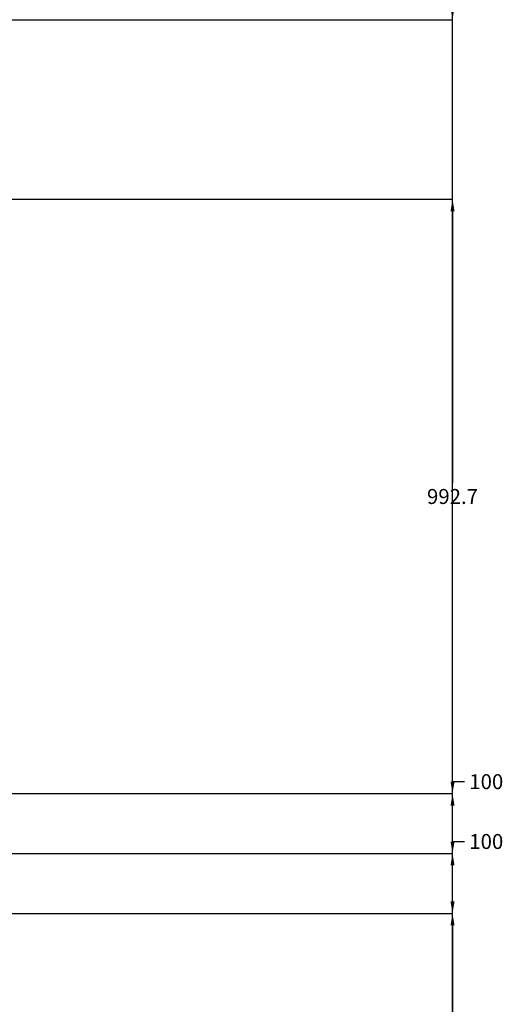
# Model space of a CAD drawing. Units: millimetres. Extents: x -692 to 9639, y -141 to 10345.
# Tile 9 of 19: x 8831 to 9639, y 1504 to 3148. Entities that reach past the tile are written whole.
import ezdxf

# ---------------------------------------------------------------- set-up
doc = ezdxf.new("R2010")
doc.units = ezdxf.units.MM
doc.header["$MEASUREMENT"] = 0
doc.layers.add('A-ANNO-DIMS', color=2, linetype='Continuous', lineweight=18)
doc.styles.get("Standard").update_dxf_attribs({"font": 'arial.ttf'})
doc.dimstyles.get("Standard").update_dxf_attribs({"dimtxt": 25, "dimasz": 20, "dimexe": 0.18, "dimexo": 10, "dimgap": 10, "dimtad": 0, "dimtih": 1, "dimtoh": 1, "dimdec": 0, "dimzin": 0, "dimdsep": 46, "dimtxsty": 'Standard', "dimcen": 10, "dimadec": 0, "dimazin": 0, "dimtfac": 1, "dimtdec": 0, "dimtofl": 0, "dimtmove": 0, "dimatfit": 3, "dimfxl": 1, "dimtolj": 1, "dimtzin": 0, "dimarcsym": 0})

# ---------------------------------------------------------------- blocks, each defined once
blk = doc.blocks.new('*D9')
at = {"layer": 'A-ANNO-DIMS', "color": 0, "lineweight": -2, "transparency": 16777216}
for p, q in [((8501.5, 8848.8), (9553.9, 8848.8)), ((9553.7, 8828.8), (9553.7, 4874.9)), ((9553.7, 875.6), (9553.7, 4829.4)), ((9083.7, 855.6), (9553.9, 855.6))]:
    blk.add_line(p, q, dxfattribs=at)
at = {"layer": 'A-ANNO-DIMS', "color": 0, "lineweight": -3, "transparency": 16777216}
for points in [[(9550.4, 8828.8), (9557.1, 8828.8), (9553.7, 8848.8)], [(9550.4, 875.6), (9557.1, 875.6), (9553.7, 855.6)]]:
    blk.add_solid(points, dxfattribs=at)
at = {"layer": 'Defpoints', "color": 0, "lineweight": -3, "transparency": 16777216}
for p in [(8491.5, 8848.8), (9553.7, 8848.8), (9073.7, 855.6)]:
    blk.add_point(p, dxfattribs=at)
at = {"layer": 'A-ANNO-DIMS', "color": 0, "transparency": 16777216, "insert": (9553.7, 4852.2), "char_height": 25, "attachment_point": 5}
blk.add_mtext('\\A1;7993', dxfattribs=at)
blk = doc.blocks.new('*D28')
at = {"layer": 'A-ANNO-DIMS', "color": 0, "lineweight": -2, "transparency": 16777216}
for p, q in [((8583.7, 1655.6), (9553.9, 1655.6)), ((9553.7, 1635.6), (9553.7, 1278.3)), ((9553.7, 875.6), (9553.7, 1232.8)), ((8583.7, 855.6), (9553.9, 855.6))]:
    blk.add_line(p, q, dxfattribs=at)
at = {"layer": 'A-ANNO-DIMS', "color": 0, "lineweight": -3, "transparency": 16777216}
for points in [[(9550.4, 1635.6), (9557.1, 1635.6), (9553.7, 1655.6)], [(9550.4, 875.6), (9557.1, 875.6), (9553.7, 855.6)]]:
    blk.add_solid(points, dxfattribs=at)
at = {"layer": 'Defpoints', "color": 0, "lineweight": -3, "transparency": 16777216}
for p in [(8573.7, 1655.6), (9553.7, 1655.6), (8573.7, 855.6)]:
    blk.add_point(p, dxfattribs=at)
at = {"layer": 'A-ANNO-DIMS', "color": 0, "transparency": 16777216, "insert": (9553.7, 1255.6), "char_height": 25, "attachment_point": 5}
blk.add_mtext('\\A1;800', dxfattribs=at)
blk = doc.blocks.new('*D29')
at = {"layer": 'A-ANNO-DIMS', "color": 0, "lineweight": -2, "transparency": 16777216}
for p, q in [((9553.7, 1755.6), (9553.7, 1775.6)), ((9553.7, 1775.6), (9573.7, 1775.6)), ((8683.7, 1755.6), (9553.9, 1755.6)), ((9553.7, 1675.6), (9553.7, 1735.6)), ((8583.7, 1655.6), (9553.9, 1655.6))]:
    blk.add_line(p, q, dxfattribs=at)
at = {"layer": 'A-ANNO-DIMS', "color": 0, "lineweight": -3, "transparency": 16777216}
for points in [[(9550.4, 1735.6), (9557.1, 1735.6), (9553.7, 1755.6)], [(9550.4, 1675.6), (9557.1, 1675.6), (9553.7, 1655.6)]]:
    blk.add_solid(points, dxfattribs=at)
at = {"layer": 'Defpoints', "color": 0, "lineweight": -3, "transparency": 16777216}
for p in [(8673.7, 1755.6), (9553.7, 1755.6), (8573.7, 1655.6)]:
    blk.add_point(p, dxfattribs=at)
at = {"layer": 'A-ANNO-DIMS', "color": 0, "transparency": 16777216, "insert": (9610.1, 1775.6), "char_height": 25, "attachment_point": 5}
blk.add_mtext('\\A1;100', dxfattribs=at)
blk = doc.blocks.new('*D30')
at = {"layer": 'A-ANNO-DIMS', "color": 0, "lineweight": -2, "transparency": 16777216}
for p, q in [((9553.7, 1855.6), (9553.7, 1875.6)), ((9553.7, 1875.6), (9573.7, 1875.6)), ((8783.7, 1855.6), (9553.9, 1855.6)), ((9553.7, 1775.6), (9553.7, 1835.6)), ((8683.7, 1755.6), (9553.9, 1755.6))]:
    blk.add_line(p, q, dxfattribs=at)
at = {"layer": 'A-ANNO-DIMS', "color": 0, "lineweight": -3, "transparency": 16777216}
for points in [[(9550.4, 1835.6), (9557.1, 1835.6), (9553.7, 1855.6)], [(9550.4, 1775.6), (9557.1, 1775.6), (9553.7, 1755.6)]]:
    blk.add_solid(points, dxfattribs=at)
at = {"layer": 'Defpoints', "color": 0, "lineweight": -3, "transparency": 16777216}
for p in [(8773.7, 1855.6), (9553.7, 1855.6), (8673.7, 1755.6)]:
    blk.add_point(p, dxfattribs=at)
at = {"layer": 'A-ANNO-DIMS', "color": 0, "transparency": 16777216, "insert": (9610.1, 1875.6), "char_height": 25, "attachment_point": 5}
blk.add_mtext('\\A1;100', dxfattribs=at)
blk = doc.blocks.new('*D31')
at = {"layer": 'A-ANNO-DIMS', "color": 0, "lineweight": -2, "transparency": 16777216}
for p, q in [((8351.5, 2848.3), (9553.9, 2848.3)), ((9553.7, 2828.3), (9553.7, 2374.7)), ((9553.7, 1875.6), (9553.7, 2329.2)), ((8783.7, 1855.6), (9553.9, 1855.6))]:
    blk.add_line(p, q, dxfattribs=at)
at = {"layer": 'A-ANNO-DIMS', "color": 0, "lineweight": -3, "transparency": 16777216}
for points in [[(9550.4, 2828.3), (9557.1, 2828.3), (9553.7, 2848.3)], [(9550.4, 1875.6), (9557.1, 1875.6), (9553.7, 1855.6)]]:
    blk.add_solid(points, dxfattribs=at)
at = {"layer": 'Defpoints', "color": 0, "lineweight": -3, "transparency": 16777216}
for p in [(8341.5, 2848.3), (9553.7, 2848.3), (8773.7, 1855.6)]:
    blk.add_point(p, dxfattribs=at)
at = {"layer": 'A-ANNO-DIMS', "color": 0, "transparency": 16777216, "insert": (9553.7, 2351.9), "char_height": 25, "attachment_point": 5}
blk.add_mtext('\\A1;992.7', dxfattribs=at)
blk = doc.blocks.new('*D71')
at = {"layer": 'A-ANNO-DIMS', "color": 0, "lineweight": -2, "transparency": 16777216}
for p, q in [((5201.5, 3598.3), (9553.9, 3598.3)), ((9553.7, 3578.3), (9553.7, 3396)), ((9553.7, 3168.3), (9553.7, 3350.5)), ((5101.5, 3148.3), (9553.9, 3148.3))]:
    blk.add_line(p, q, dxfattribs=at)
at = {"layer": 'A-ANNO-DIMS', "color": 0, "lineweight": -3, "transparency": 16777216}
for points in [[(9550.4, 3578.3), (9557.1, 3578.3), (9553.7, 3598.3)], [(9550.4, 3168.3), (9557.1, 3168.3), (9553.7, 3148.3)]]:
    blk.add_solid(points, dxfattribs=at)
at = {"layer": 'Defpoints', "color": 0, "lineweight": -3, "transparency": 16777216}
for p in [(5191.5, 3598.3), (9553.7, 3598.3), (5091.5, 3148.3)]:
    blk.add_point(p, dxfattribs=at)
at = {"layer": 'A-ANNO-DIMS', "color": 0, "transparency": 16777216, "insert": (9553.7, 3373.3), "char_height": 25, "attachment_point": 5}
blk.add_mtext('\\A1;450', dxfattribs=at)

msp = doc.modelspace()

# ---------------------------------------------------------------- dimensions: what is measured, and where the dimension line sits
at = {"layer": 'A-ANNO-DIMS'}
for base, p1, p2, override, picture, middle in [((9553.746, 8848.772), (9073.746, 855.575), (8491.547, 8848.772), {"dimdec": 0, "dimlfac": 1, "dimrnd": 0, "dimzin": 0, "dimdsep": 46, "dimlunit": 2}, '*D9', (9553.746, 4852.173)), ((9553.746, 3598.27), (5091.547, 3148.27), (5191.547, 3598.27), {"dimdec": 0, "dimlfac": 1, "dimrnd": 0, "dimzin": 0, "dimdsep": 46, "dimlunit": 2}, '*D71', (9553.746, 3373.27)), ((9553.746, 2848.27), (8773.746, 1855.575), (8341.547, 2848.27), {"dimdec": 1, "dimlfac": 1, "dimrnd": 0, "dimzin": 0, "dimdsep": 46, "dimlunit": 2}, '*D31', (9553.746, 2351.922)), ((9553.746, 1855.575), (8673.746, 1755.575), (8773.746, 1855.575), {"dimdec": 0, "dimlfac": 1, "dimrnd": 0, "dimzin": 0, "dimdsep": 46, "dimlunit": 2}, '*D30', (9610.144, 1875.575)), ((9553.746, 1755.575), (8573.746, 1655.575), (8673.746, 1755.575), {"dimdec": 0, "dimlfac": 1, "dimrnd": 0, "dimzin": 0, "dimdsep": 46, "dimlunit": 2}, '*D29', (9610.144, 1775.575)), ((9553.746, 1655.575), (8573.746, 855.575), (8573.746, 1655.575), {"dimdec": 0, "dimlfac": 1, "dimrnd": 0, "dimzin": 0, "dimdsep": 46, "dimlunit": 2}, '*D28', (9553.746, 1255.575))]:
    dim = msp.add_linear_dim(base=base, p1=p1, p2=p2, angle=90, dimstyle='Standard', override=override, dxfattribs=at)
    dim.commit()
    dim.dimension.update_dxf_attribs({"geometry": picture, "text_midpoint": middle})

doc.saveas('drawing.dxf')
